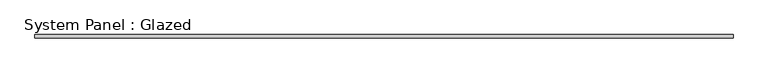
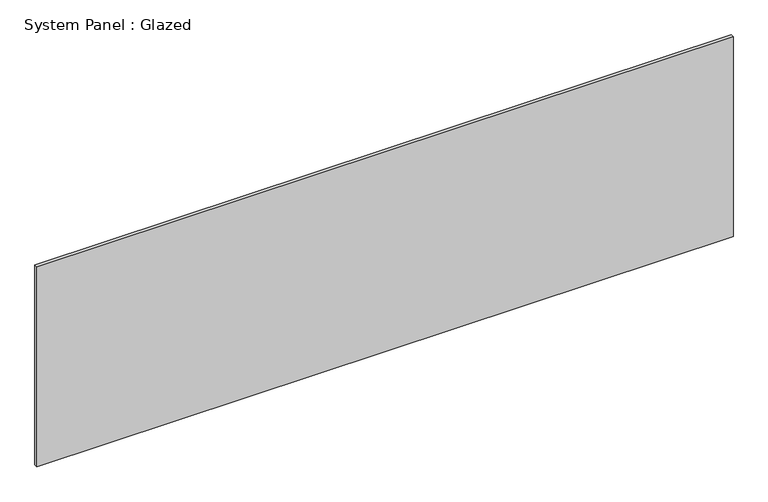
"""IFC4 building model written with IfcOpenShell, lengths in millimetres: plate geometry, System Panel : Glazed."""

from ifc_helpers import new_model, si_unit, origin, origin_with_axes, place, context, project, spatial, polyline, outline, extrude, source, transform, mapped, element, save


def system_panel_glazed_79055968(model_context):
    return source(origin(), model_context, "Body", "SweptSolid", [
        extrude(outline(polyline([(2511.601725, 19.05), (-2511.601725, 19.05), (-2511.601725, 44.45), (2511.601725, 44.45), (2511.601725, 19.05)])), origin_with_axes(), (0.0, 0.0, 1.0), 1524.0),
    ])


if __name__ == "__main__":
    model = new_model("IFC4")
    model_context = context("Model", 3, world=origin())
    ifc_project = project(units=[si_unit("LENGTHUNIT", "METRE", prefix="MILLI")], contexts=[model_context])
    site = spatial("IfcSite", under=ifc_project)
    building = spatial("IfcBuilding", under=site)
    placement = place(None, origin())
    system_panel_glazed_shape = system_panel_glazed_79055968(model_context)
    element("IfcPlate", 1, ObjectType="System Panel : Glazed", at=placement, inside=building, context=model_context, shape_type="MappedRepresentation", body=[
        mapped(system_panel_glazed_shape, transform((0.0, 0.0, 0.0), x_axis=(1.0, 0.0, 0.0), y_axis=(0.0, 1.0, 0.0), z_axis=(0.0, 0.0, 1.0))),
    ])
    save(model, "model.ifc")

# Revit data of these elements
# Type "System Panel : Glazed"
#   Construction Type Id = "GSP4R"
#   Analytic Construction = "1/8 in Pilkington single glazing"
#   Visual Light Transmittance = 0.9
#   Solar Heat Gain Coefficient = 0.86
#   Heat Transfer Coefficient (U) = 1.18115 BTU/(h·ft²·°F)
# Element 1 (IfcPlate, "System Panel : Glazed")
#   Materials on its faces: "Glass"
# Materials
#   "Glass": class "Glass", colour RGB 0 128 192, transparency 0.75, Description = "Soda Lime Glass", Cost = 0
